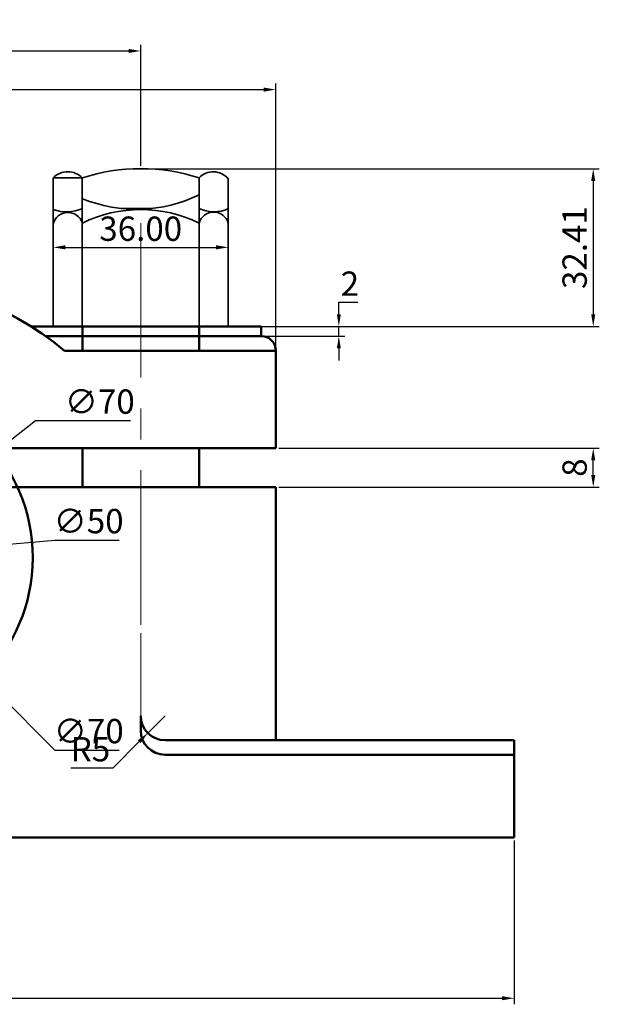
# Model space of a CAD drawing. Units: millimetres. Extents: x 2310 to 2633, y 1180 to 1382.
# Tile 2 of 2: x 2514 to 2633, y 1180 to 1382. Entities that reach past the tile are written whole.
import ezdxf

# ---------------------------------------------------------------- set-up
doc = ezdxf.new("R2010")
doc.units = ezdxf.units.MM
doc.linetypes.add('CENTER', pattern=[50.8, 31.75, -6.35, 6.35, -6.35])
for name, color, linetype, lineweight in [('M-CNTR', 1, 'CENTER', 18), ('M-DIMS', 2, 'Continuous', 25), ('M-FAST', 4, 'Continuous', 35), ('M-OUTL', 7, 'Continuous', 50)]:
    doc.layers.add(name, color=color, linetype=linetype, lineweight=lineweight)
doc.styles.get("Standard").update_dxf_attribs({"font": 'arial.ttf'})
doc.dimstyles.new('ISO-25', dxfattribs={"dimtxt": 5, "dimasz": 2.5, "dimexe": 1.25, "dimexo": 0.625, "dimtad": 1, "dimtoh": 1, "dimdec": 0, "dimtxsty": 'Standard', "dimcen": 2.5, "dimadec": 0, "dimazin": 0, "dimtfac": 1, "dimtdec": 0, "dimtmove": 0, "dimatfit": 3, "dimfxl": 1, "dimarcsym": 0})

# ---------------------------------------------------------------- blocks, each defined once
blk = doc.blocks.new('*D1')
at = {"layer": 'Defpoints', "color": 0, "transparency": 16777216}
for p in [(2538.53, 1375.88), (2424.11, 1351.69), (2538.53, 1351.69)]:
    blk.add_point(p, dxfattribs=at)
at = {"layer": 'M-DIMS', "color": 0, "lineweight": -2, "transparency": 16777216}
for p, q in [((2424.11, 1352.31), (2424.11, 1377.13)), ((2426.61, 1375.88), (2536.03, 1375.88)), ((2538.53, 1352.31), (2538.53, 1377.13))]:
    blk.add_line(p, q, dxfattribs=at)
at = {"layer": 'M-DIMS', "color": 0, "transparency": 16777216}
for points in [[(2426.61, 1376.3), (2426.61, 1375.47), (2424.11, 1375.88)], [(2536.03, 1376.3), (2536.03, 1375.47), (2538.53, 1375.88)]]:
    blk.add_solid(points, dxfattribs=at)
at = {"layer": 'M-DIMS', "color": 0, "transparency": 16777216, "insert": (2481.32, 1379.02), "char_height": 5, "attachment_point": 5}
blk.add_mtext('114', dxfattribs=at)
blk = doc.blocks.new('*D2')
at = {"layer": 'Defpoints', "color": 0, "transparency": 16777216}
for p in [(2347.32, 1214.28), (2615.32, 1214.28), (2615.32, 1181.26)]:
    blk.add_point(p, dxfattribs=at)
at = {"layer": 'M-DIMS', "color": 0, "lineweight": -2, "transparency": 16777216}
for p, q in [((2347.32, 1213.66), (2347.32, 1180.01)), ((2615.32, 1213.66), (2615.32, 1180.01)), ((2349.82, 1181.26), (2612.82, 1181.26))]:
    blk.add_line(p, q, dxfattribs=at)
at = {"layer": 'M-DIMS', "color": 0, "transparency": 16777216}
for points in [[(2349.82, 1181.68), (2349.82, 1180.85), (2347.32, 1181.26)], [(2612.82, 1181.68), (2612.82, 1180.85), (2615.32, 1181.26)]]:
    blk.add_solid(points, dxfattribs=at)
at = {"layer": 'M-DIMS', "color": 0, "transparency": 16777216, "insert": (2481.32, 1184.44), "char_height": 5, "attachment_point": 5}
blk.add_mtext('268', dxfattribs=at)
blk = doc.blocks.new('*D7')
at = {"layer": 'Defpoints', "color": 0, "transparency": 16777216}
for p in [(2563.32, 1319.28), (2579.26, 1319.28), (2563.32, 1317.28)]:
    blk.add_point(p, dxfattribs=at)
at = {"layer": 'M-DIMS', "color": 0, "lineweight": -2, "transparency": 16777216}
for p, q in [((2579.26, 1321.78), (2579.26, 1324.28)), ((2579.26, 1324.28), (2583.2, 1324.28)), ((2563.95, 1319.28), (2580.51, 1319.28)), ((2579.26, 1317.28), (2579.26, 1319.28)), ((2563.95, 1317.28), (2580.51, 1317.28)), ((2579.26, 1314.78), (2579.26, 1312.28))]:
    blk.add_line(p, q, dxfattribs=at)
at = {"layer": 'M-DIMS', "color": 0, "transparency": 16777216}
for points in [[(2578.85, 1321.78), (2579.68, 1321.78), (2579.26, 1319.28)], [(2578.85, 1314.78), (2579.68, 1314.78), (2579.26, 1317.28)]]:
    blk.add_solid(points, dxfattribs=at)
at = {"layer": 'M-DIMS', "color": 0, "transparency": 16777216, "insert": (2581.54, 1327.42), "char_height": 5, "attachment_point": 5}
blk.add_mtext('2', dxfattribs=at)
blk = doc.blocks.new('*D9')
at = {"layer": 'Defpoints', "color": 0, "transparency": 16777216}
for p in [(2508.79, 1293.47), (2453.85, 1250.09)]:
    blk.add_point(p, dxfattribs=at)
at = {"layer": 'M-DIMS', "color": 0, "lineweight": -2, "transparency": 16777216}
for p, q in [((2516.9, 1299.87), (2510.75, 1295.02)), ((2536.4, 1299.87), (2516.9, 1299.87)), ((2453.85, 1250.09), (2508.79, 1293.47)), ((2451.89, 1248.54), (2449.93, 1246.99))]:
    blk.add_line(p, q, dxfattribs=at)
at = {"layer": 'M-DIMS', "color": 0, "transparency": 16777216}
for points in [[(2510.49, 1295.35), (2511.01, 1294.69), (2508.79, 1293.47)], [(2451.63, 1248.87), (2452.15, 1248.21), (2453.85, 1250.09)]]:
    blk.add_solid(points, dxfattribs=at)
at = {"layer": 'M-DIMS', "color": 0, "transparency": 16777216, "insert": (2530.11, 1303.19), "char_height": 5, "attachment_point": 5}
blk.add_mtext('∅70', dxfattribs=at)
blk = doc.blocks.new('*D11')
at = {"layer": 'Defpoints', "color": 0, "transparency": 16777216}
for p in [(2506.22, 1274.01), (2456.42, 1269.55)]:
    blk.add_point(p, dxfattribs=at)
at = {"layer": 'M-DIMS', "color": 0, "lineweight": -2, "transparency": 16777216}
for p, q in [((2520.89, 1275.32), (2508.71, 1274.23)), ((2534.1, 1275.32), (2520.89, 1275.32)), ((2456.42, 1269.55), (2506.22, 1274.01)), ((2453.93, 1269.33), (2451.44, 1269.11))]:
    blk.add_line(p, q, dxfattribs=at)
at = {"layer": 'M-DIMS', "color": 0, "transparency": 16777216}
for points in [[(2508.68, 1274.64), (2508.75, 1273.81), (2506.22, 1274.01)], [(2453.89, 1269.75), (2453.97, 1268.92), (2456.42, 1269.55)]]:
    blk.add_solid(points, dxfattribs=at)
at = {"layer": 'M-DIMS', "color": 0, "transparency": 16777216, "insert": (2527.81, 1278.64), "char_height": 5, "attachment_point": 5}
blk.add_mtext('∅50', dxfattribs=at)
blk = doc.blocks.new('HEX-NUT-M16')
for p, q in [((6.01, 27.03), (6.01, 30.51)), ((30.01, 30.51), (36.01, 30.51)), ((30.01, 28.24), (30.01, 30.51)), ((36.01, 28), (36.01, 30.51)), ((0.01, 21.24), (0.01, 30.34)), ((6.01, 24.24), (6.01, 27.03)), ((30.01, 24.24), (30.01, 28.24)), ((36.01, 24), (36.01, 28)), ((6.01, 21.24), (6.01, 24.24)), ((22, 24.24), (15.78, 24.24)), ((30.01, 21.24), (30.01, 24.24)), ((36.01, 21), (36.01, 24)), ((0.01, 0), (0.01, 21.24)), ((6.01, 21.24), (6.01, 0)), ((30.01, 21.24), (30.01, 0)), ((36.01, 0), (36.01, 21)), ((6.01, 0), (0.01, 0)), ((30.01, 0), (36.01, 0))]:
    blk.add_line(p, q)
for centre, radius, start, end in [((18.01, -6.51), 38.92, 72.0429, 107.9571), ((3.08, 27.76), 4.01, 43.2858, 140.0947), ((33.01, 27.59), 4.19, 44.2799, 135.7201), ((18.89, 53.7), 29.62, 244.2052, 292.0376), ((2.96, 30.62), 7.07, 245.1977, 295.4854), ((3.01, 20.39), 3.12, 15.8422, 164.1674), ((18.01, -3.45), 27.45, 64.08, 115.92), ((33.32, 31.95), 8.39, 246.714, 288.6385), ((32.97, 20.31), 3.11, 12.8097, 162.5427)]:
    blk.add_arc(centre, radius, start, end)
blk = doc.blocks.new('*D13')
at = {"layer": 'Defpoints', "color": 0, "transparency": 16777216}
for p in [(2566.32, 1367.94), (2396.32, 1314.28), (2566.32, 1314.28)]:
    blk.add_point(p, dxfattribs=at)
at = {"layer": 'M-DIMS', "color": 0, "lineweight": -2, "transparency": 16777216}
for p, q in [((2396.32, 1314.91), (2396.32, 1369.19)), ((2398.82, 1367.94), (2563.82, 1367.94)), ((2566.32, 1314.91), (2566.32, 1369.19))]:
    blk.add_line(p, q, dxfattribs=at)
at = {"layer": 'M-DIMS', "color": 0, "transparency": 16777216}
for points in [[(2398.82, 1368.36), (2398.82, 1367.52), (2396.32, 1367.94)], [(2563.82, 1368.36), (2563.82, 1367.52), (2566.32, 1367.94)]]:
    blk.add_solid(points, dxfattribs=at)
at = {"layer": 'M-DIMS', "color": 0, "transparency": 16777216, "insert": (2481.32, 1371.12), "char_height": 5, "attachment_point": 5}
blk.add_mtext('170', dxfattribs=at)
blk = doc.blocks.new('*D14')
at = {"layer": 'Defpoints', "color": 0, "transparency": 16777216}
for p in [(2566.32, 1294.28), (2631.57, 1294.28), (2566.32, 1286.28)]:
    blk.add_point(p, dxfattribs=at)
at = {"layer": 'M-DIMS', "color": 0, "lineweight": -2, "transparency": 16777216}
for p, q in [((2566.95, 1294.28), (2632.82, 1294.28)), ((2631.57, 1288.78), (2631.57, 1291.78)), ((2566.95, 1286.28), (2632.82, 1286.28))]:
    blk.add_line(p, q, dxfattribs=at)
at = {"layer": 'M-DIMS', "color": 0, "transparency": 16777216}
for points in [[(2631.15, 1291.78), (2631.99, 1291.78), (2631.57, 1294.28)], [(2631.15, 1288.78), (2631.99, 1288.78), (2631.57, 1286.28)]]:
    blk.add_solid(points, dxfattribs=at)
at = {"layer": 'M-DIMS', "color": 0, "transparency": 16777216, "insert": (2628.39, 1290.28), "char_height": 5, "attachment_point": 5, "rotation": 90}
blk.add_mtext('8', dxfattribs=at)
blk = doc.blocks.new('*D15')
at = {"layer": 'Defpoints', "color": 0, "transparency": 16777216}
for p in [(2538.53, 1351.69), (2556.53, 1319.28), (2631.57, 1319.28)]:
    blk.add_point(p, dxfattribs=at)
at = {"layer": 'M-DIMS', "color": 0, "lineweight": -2, "transparency": 16777216}
for p, q in [((2539.15, 1351.69), (2632.82, 1351.69)), ((2631.57, 1349.19), (2631.57, 1321.78)), ((2557.15, 1319.28), (2632.82, 1319.28))]:
    blk.add_line(p, q, dxfattribs=at)
at = {"layer": 'M-DIMS', "color": 0, "transparency": 16777216}
for points in [[(2631.15, 1349.19), (2631.99, 1349.19), (2631.57, 1351.69)], [(2631.15, 1321.78), (2631.99, 1321.78), (2631.57, 1319.28)]]:
    blk.add_solid(points, dxfattribs=at)
at = {"layer": 'M-DIMS', "color": 0, "transparency": 16777216, "insert": (2628.39, 1335.48), "char_height": 5, "attachment_point": 5, "rotation": 90}
blk.add_mtext('32.41', dxfattribs=at)
blk = doc.blocks.new('*D20')
at = {"layer": 'Defpoints', "color": 0, "transparency": 16777216}
for p in [(2456.57, 1296.53), (2506.07, 1247.03)]:
    blk.add_point(p, dxfattribs=at)
at = {"layer": 'M-DIMS', "color": 0, "lineweight": -2, "transparency": 16777216}
for p, q in [((2454.81, 1298.3), (2453.04, 1300.07)), ((2456.57, 1296.53), (2506.07, 1247.03)), ((2520.92, 1232.18), (2507.84, 1245.26)), ((2534.13, 1232.18), (2520.92, 1232.18))]:
    blk.add_line(p, q, dxfattribs=at)
at = {"layer": 'M-DIMS', "color": 0, "transparency": 16777216}
for points in [[(2455.1, 1298.59), (2454.51, 1298), (2456.57, 1296.53)], [(2508.13, 1245.56), (2507.54, 1244.97), (2506.07, 1247.03)]]:
    blk.add_solid(points, dxfattribs=at)
at = {"layer": 'M-DIMS', "color": 0, "transparency": 16777216, "insert": (2527.84, 1235.5), "char_height": 5, "attachment_point": 5}
blk.add_mtext('∅70', dxfattribs=at)
blk = doc.blocks.new('*D22')
at = {"layer": 'Defpoints', "color": 0, "transparency": 16777216}
for p in [(2543.53, 1239.28), (2539.99, 1235.74)]:
    blk.add_point(p, dxfattribs=at)
at = {"layer": 'M-DIMS', "color": 0, "lineweight": -2, "transparency": 16777216}
for p, q in [((2543.53, 1239.28), (2539.99, 1235.74)), ((2532.86, 1228.61), (2538.23, 1233.98)), ((2524.14, 1228.61), (2532.86, 1228.61))]:
    blk.add_line(p, q, dxfattribs=at)
at = {"layer": 'M-DIMS', "color": 0, "transparency": 16777216}
blk.add_solid([(2537.93, 1234.27), (2538.52, 1233.68), (2539.99, 1235.74)], dxfattribs=at)
at = {"layer": 'M-DIMS', "color": 0, "transparency": 16777216, "insert": (2528.19, 1231.78), "char_height": 5, "attachment_point": 5}
blk.add_mtext('R5', dxfattribs=at)
blk = doc.blocks.new('*D24')
at = {"layer": 'Defpoints', "color": 0, "transparency": 16777216}
for p in [(2556.53, 1335.53), (2520.53, 1319.28), (2556.53, 1319.28)]:
    blk.add_point(p, dxfattribs=at)
at = {"layer": 'M-DIMS', "color": 0, "lineweight": -2, "transparency": 16777216}
for p, q in [((2520.53, 1319.91), (2520.53, 1336.78)), ((2523.03, 1335.53), (2554.03, 1335.53)), ((2556.53, 1319.91), (2556.53, 1336.78))]:
    blk.add_line(p, q, dxfattribs=at)
at = {"layer": 'M-DIMS', "color": 0, "transparency": 16777216}
for points in [[(2523.03, 1335.95), (2523.03, 1335.11), (2520.53, 1335.53)], [(2554.03, 1335.95), (2554.03, 1335.11), (2556.53, 1335.53)]]:
    blk.add_solid(points, dxfattribs=at)
at = {"layer": 'M-DIMS', "color": 0, "transparency": 16777216, "insert": (2538.53, 1338.71), "char_height": 5, "attachment_point": 5}
blk.add_mtext('36.00', dxfattribs=at)

msp = doc.modelspace()

# ---------------------------------------------------------------- linework, layer by layer
at = {"layer": 'M-CNTR'}
for p, q in [((2538.5284, 1340.5239), (2538.5284, 1256.2344)), ((2538.5284, 1256.2344), (2538.5284, 1239.2804))]:
    msp.add_line(p, q, dxfattribs=at)
at = {"layer": 'M-OUTL'}
for p, q in [((2563.3215, 1319.2804), (2515.9625, 1319.2804)), ((2515.9625, 1319.2804), (2563.3215, 1319.2804)), ((2526.5284, 1319.2804), (2526.5284, 1314.2804)), ((2550.5284, 1319.2804), (2550.5284, 1314.2804)), ((2563.3215, 1317.2804), (2563.3215, 1319.2804)), ((2563.3215, 1317.2804), (2518.9512, 1317.2804)), ((2566.3215, 1314.2804), (2522.8546, 1314.2804)), ((2566.3215, 1314.2804), (2522.8546, 1314.2804)), ((2566.3215, 1314.2804), (2566.3215, 1314.2804)), ((2566.3215, 1294.2804), (2566.3215, 1314.2804)), ((2396.3215, 1294.2804), (2566.3215, 1294.2804)), ((2526.5284, 1294.2804), (2526.5284, 1286.2804)), ((2550.5284, 1294.2804), (2550.5284, 1286.2804)), ((2566.3215, 1286.2804), (2396.3215, 1286.2804)), ((2566.3215, 1234.2804), (2566.3215, 1286.2804)), ((2538.5284, 1239.2804), (2538.5284, 1236.2804)), ((2566.3215, 1234.2804), (2543.5284, 1234.2804)), ((2581.3215, 1234.2804), (2566.3215, 1234.2804)), ((2615.3215, 1234.2804), (2581.3215, 1234.2804)), ((2615.3215, 1214.2804), (2615.3215, 1234.2804)), ((2615.3215, 1234.2804), (2615.3215, 1231.2804)), ((2615.3215, 1231.2804), (2543.5284, 1231.2804)), ((2347.3215, 1214.2804), (2615.3215, 1214.2804))]:
    msp.add_line(p, q, dxfattribs=at)
for centre, radius, start, end in [((2481.3215, 1264.2804), 65, 50.284863, 129.715137), ((2563.3215, 1314.2804), 3, 0, 90), ((2481.3215, 1271.7804), 35, 270, 90), ((2543.5284, 1239.2804), 5, 180, 270), ((2543.5284, 1236.2804), 5, 180, 270)]:
    msp.add_arc(centre, radius, start, end, dxfattribs=at)

# ---------------------------------------------------------------- block references
at = {"layer": 'M-FAST', "extrusion": (0, 0, -1), "zscale": -1}
msp.add_blockref('HEX-NUT-M16', (-2556.5339, 1319.28), dxfattribs=at)

# ---------------------------------------------------------------- dimensions: what is measured, and where the dimension line sits
at = {"layer": 'M-DIMS'}
for base, p1, p2, override, picture, middle in [((2538.5284, 1375.8841), (2424.1145, 1351.6891), (2538.5284, 1351.6891), {"dimclrd": 0, "dimclre": 0, "dimclrt": 0}, '*D1', (2481.3215, 1379.0193)), ((2566.3215, 1367.9391), (2396.3215, 1314.2804), (2566.3215, 1314.2804), {"dimdec": 0, "dimlfac": 1, "dimrnd": 0, "dimzin": 0, "dimdsep": 46, "dimlunit": 2}, '*D13', (2481.3215, 1371.117)), ((2556.5284, 1335.5304), (2520.5284, 1319.2804), (2556.5284, 1319.2804), {"dimdec": 2, "dimlfac": 1, "dimrnd": 0, "dimzin": 0, "dimdsep": 46, "dimlunit": 2}, '*D24', (2538.5284, 1338.71)), ((2615.3215, 1181.2637), (2347.3215, 1214.2804), (2615.3215, 1214.2804), {"dimclrd": 0, "dimclre": 0, "dimclrt": 0}, '*D2', (2481.3215, 1184.4416))]:
    dim = msp.add_linear_dim(base=base, p1=p1, p2=p2, dimstyle='ISO-25', override=override, dxfattribs=at)
    dim.commit()
    dim.dimension.update_dxf_attribs({"geometry": picture, "text_midpoint": middle})
for base, p1, p2, override, picture, middle in [((2631.5715, 1319.2804), (2538.5284, 1351.6891), (2556.5284, 1319.2804), {"dimdec": 2, "dimlfac": 1, "dimrnd": 0, "dimzin": 0, "dimdsep": 46, "dimlunit": 2}, '*D15', (2628.3919, 1335.4848)), ((2579.2638, 1319.2804), (2563.3215, 1317.2804), (2563.3215, 1319.2804), {"dimclrd": 0, "dimclre": 0, "dimclrt": 0}, '*D7', (2581.5447, 1327.4156)), ((2631.5715, 1294.2804), (2566.3215, 1286.2804), (2566.3215, 1294.2804), {"dimdec": 0, "dimlfac": 1, "dimrnd": 0, "dimzin": 0, "dimdsep": 46, "dimlunit": 2}, '*D14', (2628.3936, 1290.2804))]:
    dim = msp.add_linear_dim(base=base, p1=p1, p2=p2, angle=90, dimstyle='ISO-25', override=override, dxfattribs=at)
    dim.commit()
    dim.dimension.update_dxf_attribs({"geometry": picture, "text_midpoint": middle})
for p1, p2, override, picture, middle in [((2453.8521, 1250.0909), (2508.7908, 1293.4699), {"dimclrd": 0, "dimclre": 0, "dimclrt": 0}, '*D9', (2530.1117, 1299.8739)), ((2456.5736, 1296.53), (2506.0693, 1247.0307), {"dimdec": 0, "dimlfac": 1, "dimrnd": 0, "dimzin": 0, "dimdsep": 46, "dimlunit": 2}, '*D20', (2527.8356, 1232.1809)), ((2456.4208, 1269.5541), (2506.2221, 1274.0067), {"dimclrd": 0, "dimclre": 0, "dimclrt": 0}, '*D11', (2520.8898, 1275.3181))]:
    dim = msp.add_diameter_dim_2p(p1=p1, p2=p2, dimstyle='ISO-25', override=override, dxfattribs=at)
    dim.commit()
    dim.dimension.update_dxf_attribs({"geometry": picture, "text_midpoint": middle, "dimtype": 163})
dim = msp.add_radius_dim(center=(2543.5284, 1239.2804), mpoint=(2539.9929, 1235.7449), dimstyle='ISO-25', override={"dimdec": 0, "dimlfac": 1, "dimrnd": 0, "dimzin": 0, "dimdsep": 46, "dimlunit": 2}, dxfattribs=at)
dim.commit()
dim.dimension.update_dxf_attribs({"geometry": '*D22', "text_midpoint": (2528.1864, 1231.7811)})

doc.saveas('drawing.dxf')
